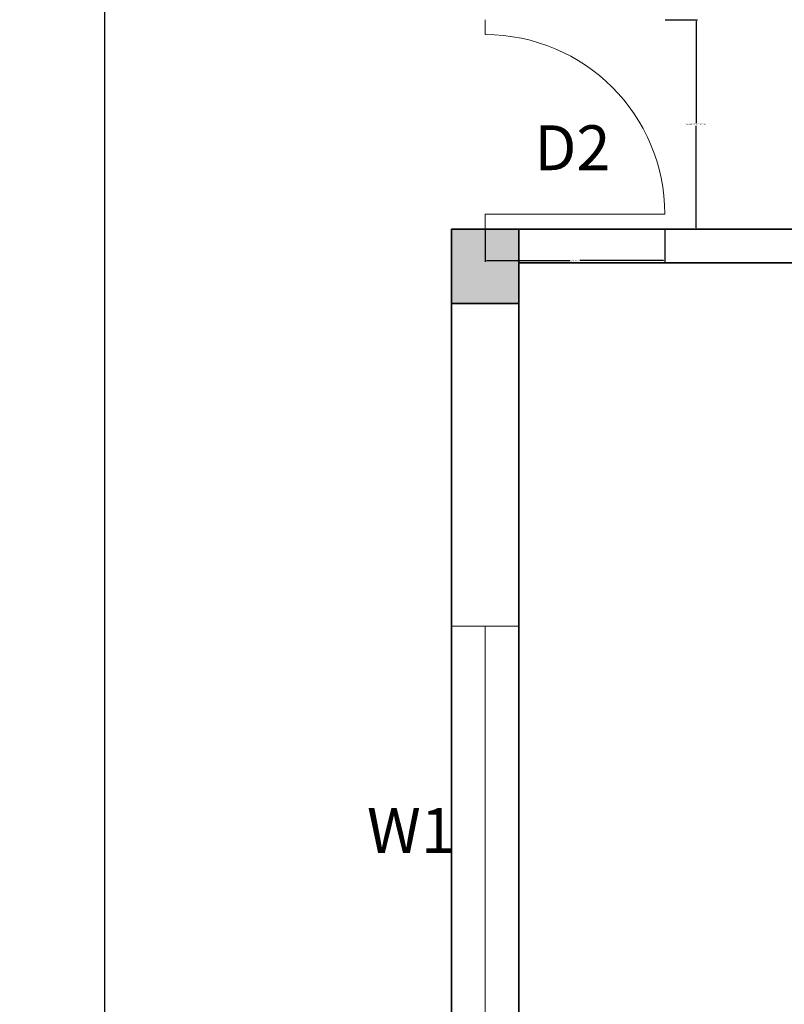
# Model space of a CAD drawing. Units: inches. Extents: x -36302355 to 648, y -221479757 to 75.
# Tile 23 of 37: x 87 to 190, y -271 to -139. Entities that reach past the tile are written whole.
import ezdxf

# ---------------------------------------------------------------- set-up
doc = ezdxf.new("R2010")
doc.units = ezdxf.units.IN
doc.header["$MEASUREMENT"] = 0
for name, color, linetype, lineweight in [('A-ANNO-DIMS', 2, 'Continuous', 18), ('A-ANNO-IDEN', 7, 'Continuous', 18), ('A-COLS', 7, 'Continuous', 35), ('A-COLS-PATT', 242, 'Continuous', 13), ('A-DOOR', 4, 'Continuous', 18), ('A-GLAZ', 142, 'Continuous', 18), ('A-WALL', 7, 'Continuous', 35)]:
    doc.layers.add(name, color=color, linetype=linetype, lineweight=lineweight)
doc.styles.get("Standard").update_dxf_attribs({"font": 'arial.ttf'})
doc.dimstyles.get("Standard").update_dxf_attribs({"dimtxt": 0.18, "dimasz": 0.18, "dimexe": 0.18, "dimexo": 0.0625, "dimgap": 0.09, "dimtad": 0, "dimtih": 1, "dimtoh": 1, "dimdec": 0, "dimzin": 0, "dimdsep": 46, "dimlunit": 3, "dimtxsty": 'Standard', "dimcen": 0.09, "dimadec": 0, "dimazin": 0, "dimtfac": 1, "dimtdec": 0, "dimtofl": 0, "dimtmove": 0, "dimatfit": 3, "dimfxl": 1, "dimtolj": 1, "dimtzin": 0, "dimarcsym": 0})

# ---------------------------------------------------------------- blocks, each defined once
blk = doc.blocks.new('*D7')
at = {"layer": 'A-ANNO-DIMS', "color": 0, "lineweight": -2, "transparency": 16777216}
for p, q in [((145.13, 24.98), (98.63, 24.98)), ((98.81, 24.8), (98.81, -274.37)), ((98.81, -579.84), (98.81, -280.67)), ((145.13, -580.02), (98.63, -580.02))]:
    blk.add_line(p, q, dxfattribs=at)
at = {"layer": 'A-ANNO-DIMS', "color": 0, "transparency": 16777216}
for points in [[(98.78, 24.8), (98.84, 24.8), (98.81, 24.98)], [(98.78, -579.84), (98.84, -579.84), (98.81, -580.02)]]:
    blk.add_solid(points, dxfattribs=at)
at = {"layer": 'Defpoints', "color": 0, "transparency": 16777216}
for p in [(98.81, 24.98), (145.2, 24.98), (145.2, -580.02)]:
    blk.add_point(p, dxfattribs=at)
at = {"layer": 'A-ANNO-DIMS', "color": 0, "transparency": 16777216, "insert": (98.81, -277.52), "char_height": 6, "attachment_point": 5}
blk.add_mtext('\\A1;50\'-5"', dxfattribs=at)
blk = doc.blocks.new('WIN-60')
for p, q in [((60, 9), (0, 9)), ((0, 9), (0, 0)), ((60, 0), (60, 9)), ((0, 4.5), (60, 4.5)), ((0, 0), (60, 0))]:
    blk.add_line(p, q)
blk = doc.blocks.new('DOOR-SWING-24')
for p, q in [((0, 26), (0, 28)), ((0, 0), (0, 2)), ((0, 2), (24, 2))]:
    blk.add_line(p, q)
blk.add_arc((0, 2), 24, 0, 90)
blk = doc.blocks.new('*D25')
at = {"layer": 'A-ANNO-DIMS', "color": 0, "lineweight": -2, "transparency": 16777216}
for p, q in [((173.76, -139.02), (178.08, -139.02)), ((177.9, -139.2), (177.9, -152.84)), ((177.9, -166.84), (177.9, -153.2)), ((173.76, -167.02), (178.08, -167.02))]:
    blk.add_line(p, q, dxfattribs=at)
at = {"layer": 'A-ANNO-DIMS', "color": 0, "transparency": 16777216}
for points in [[(177.87, -139.2), (177.93, -139.2), (177.9, -139.02)], [(177.87, -166.84), (177.93, -166.84), (177.9, -167.02)]]:
    blk.add_solid(points, dxfattribs=at)
at = {"layer": 'Defpoints', "color": 0, "transparency": 16777216}
for p in [(173.7, -139.02), (177.9, -139.02), (173.7, -167.02)]:
    blk.add_point(p, dxfattribs=at)
at = {"layer": 'A-ANNO-DIMS', "color": 0, "transparency": 16777216, "insert": (177.9, -153.02), "char_height": 0.18, "attachment_point": 5}
blk.add_mtext('\\A1;SWING DOOR 2\'-4" TYP.', dxfattribs=at)
blk = doc.blocks.new('*D26')
at = {"layer": 'A-ANNO-DIMS', "color": 0, "lineweight": -2, "transparency": 16777216}
for p, q in [((149.7, -167.08), (149.7, -171.4)), ((173.7, -167.08), (173.7, -171.4)), ((149.88, -171.22), (161.06, -171.22)), ((173.52, -171.22), (162.34, -171.22))]:
    blk.add_line(p, q, dxfattribs=at)
at = {"layer": 'A-ANNO-DIMS', "color": 0, "transparency": 16777216}
for points in [[(149.88, -171.19), (149.88, -171.25), (149.7, -171.22)], [(173.52, -171.19), (173.52, -171.25), (173.7, -171.22)]]:
    blk.add_solid(points, dxfattribs=at)
at = {"layer": 'Defpoints', "color": 0, "transparency": 16777216}
for p in [(149.7, -167.02), (173.7, -167.02), (173.7, -171.22)]:
    blk.add_point(p, dxfattribs=at)
at = {"layer": 'A-ANNO-DIMS', "color": 0, "transparency": 16777216, "insert": (161.7, -171.22), "char_height": 0.18, "attachment_point": 5}
blk.add_mtext('\\A1;2\'-0" TYP.', dxfattribs=at)

msp = doc.modelspace()

# ---------------------------------------------------------------- hatches: boundary and pattern name
at = {"layer": 'A-COLS-PATT'}
h = msp.add_hatch(color=256, dxfattribs=at)
h.dxf.hatch_style = 1
h.paths.add_polyline_path([(145.2, 24.98), (145.2, 15.98), (154.2, 15.98), (154.2, 24.98)])
h.paths.add_polyline_path([(247.2, 15.98), (247.2, 24.98), (238.2, 24.98), (238.2, 15.98)])
h.paths.add_polyline_path([(387.64, 15.98), (395.7, 15.98), (395.7, 24.98), (387.64, 24.98)])
h.paths.add_polyline_path([(451.26, 24.98), (443.7, 24.98), (443.7, 15.98), (451.26, 15.98)])
h.paths.add_polyline_path([(596.2, 15.98), (605.2, 15.98), (605.2, 24.98), (596.2, 24.98)])
h.paths.add_polyline_path([(238.2, -122.02), (238.2, -131.02), (247.2, -131.02), (247.2, -122.02)])
h.paths.add_polyline_path([(395.7, -122.02), (387.46, -122.02), (387.46, -131.02), (395.7, -131.02)])
h.paths.add_polyline_path([(448.2, -131.02), (453.73, -131.02), (453.73, -122.02), (443.7, -122.02), (443.7, -131.02)])
h.paths.add_polyline_path([(596.2, -131.02), (605.2, -131.02), (605.2, -122.02), (596.2, -122.02)])
h.paths.add_polyline_path([(145.2, -176.97), (154.2, -176.97), (154.2, -167.02), (145.2, -167.02)])
h.paths.add_polyline_path([(314.2, -176.97), (323.2, -176.97), (323.2, -167.02), (314.2, -167.02)])
h.paths.add_polyline_path([(154.2, -314.02), (154.2, -309.52), (145.2, -309.52), (145.2, -314.02)])
h.paths.add_polyline_path([(314.2, -309.52), (314.2, -318.52), (323.2, -318.52), (323.2, -309.52)])
h.paths.add_polyline_path([(448.2, -277.02), (443.7, -277.02), (443.7, -286.02), (448.2, -286.02)])
h.paths.add_polyline_path([(283.2, -370.02), (274.2, -370.02), (274.2, -379.02), (283.2, -379.02), (283.2, -374.52)])
h.paths.add_polyline_path([(154.2, -370.02), (145.2, -370.02), (145.2, -379.02), (154.2, -379.02)])
h.paths.add_polyline_path([(443.2, -374.52), (443.2, -379.02), (452.2, -379.02), (452.2, -374.52)])
h.paths.add_polyline_path([(145.2, -580.02), (154.2, -580.02), (154.2, -571.02), (145.2, -571.02)])
h.paths.add_polyline_path([(274.2, -571.02), (274.2, -580.02), (283.2, -580.02), (283.2, -571.02)])
h.paths.add_polyline_path([(443.2, -580.02), (452.2, -580.02), (452.2, -571.02), (443.2, -571.02)])

# ---------------------------------------------------------------- linework, layer by layer
at = {"layer": 'A-COLS'}
for p, q in [((145.2, -167.02), (145.2, -167.02)), ((147.53, -176.97), (145.2, -176.97)), ((145.2, -176.97), (154.2, -176.97))]:
    msp.add_line(p, q, dxfattribs=at)
at = {"layer": 'A-WALL'}
for p, q in [((145.2, -167.02), (323.2, -167.02)), ((145.2, -167.02), (145.2, -722.02)), ((154.2, -167.02), (154.2, -722.02)), ((154.2, -171.52), (314.2, -171.52))]:
    msp.add_line(p, q, dxfattribs=at)

# ---------------------------------------------------------------- block references
at = {"layer": 'A-DOOR'}
msp.add_blockref('DOOR-SWING-24', (149.7, -167.02), dxfattribs=at)
at = {"layer": 'A-GLAZ', "extrusion": (0, 0, -1), "zscale": -1, "rotation": 90}
msp.add_blockref('WIN-60', (-145.2, -280.1), dxfattribs=at)

# ---------------------------------------------------------------- texts
at = {"layer": 'A-ANNO-IDEN', "insert": (156.27, -153.14), "char_height": 6, "attachment_point": 1}
msp.add_mtext('D2', dxfattribs=at)
at = {"layer": 'A-ANNO-IDEN', "insert": (133.91, -244.43), "char_height": 6, "attachment_point": 1}
msp.add_mtext_dynamic_manual_height_columns('W1', width=0.8021, gutter_width=1, heights=[0], dxfattribs=at)

# ---------------------------------------------------------------- dimensions: what is measured, and where the dimension line sits
at = {"layer": 'A-ANNO-DIMS'}
dim = msp.add_linear_dim(base=(98.81, 24.98), p1=(145.2, -580.02), p2=(145.2, 24.98), angle=90, dimstyle='Standard', override={"dimtxt": 6, "dimclrd": 0, "dimclre": 0, "dimclrt": 0}, dxfattribs=at)
dim.commit()
dim.dimension.update_dxf_attribs({"geometry": '*D7', "text_midpoint": (98.81, -277.52)})
dim = msp.add_linear_dim(base=(177.9, -139.02), p1=(173.7, -167.02), p2=(173.7, -139.02), angle=90, text='SWING DOOR <> TYP.', dimstyle='Standard', override={"dimdec": 1, "dimlfac": 1, "dimrnd": 0, "dimzin": 1, "dimdsep": 46, "dimlunit": 4, "dimfrac": 2}, dxfattribs=at)
dim.commit()
dim.dimension.update_dxf_attribs({"geometry": '*D25', "text_midpoint": (177.9, -153.02)})
dim = msp.add_linear_dim(base=(173.7, -171.22), p1=(149.7, -167.02), p2=(173.7, -167.02), text='<> TYP.', dimstyle='Standard', override={"dimdec": 1, "dimlfac": 1, "dimrnd": 0, "dimzin": 1, "dimdsep": 46, "dimlunit": 4, "dimfrac": 2}, dxfattribs=at)
dim.commit()
dim.dimension.update_dxf_attribs({"geometry": '*D26', "text_midpoint": (161.7, -171.22)})

doc.saveas('drawing.dxf')
